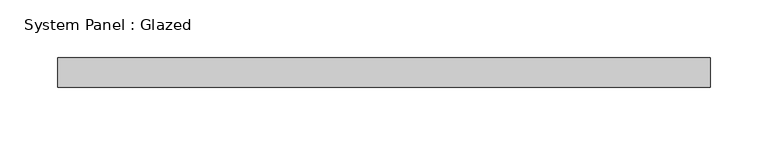
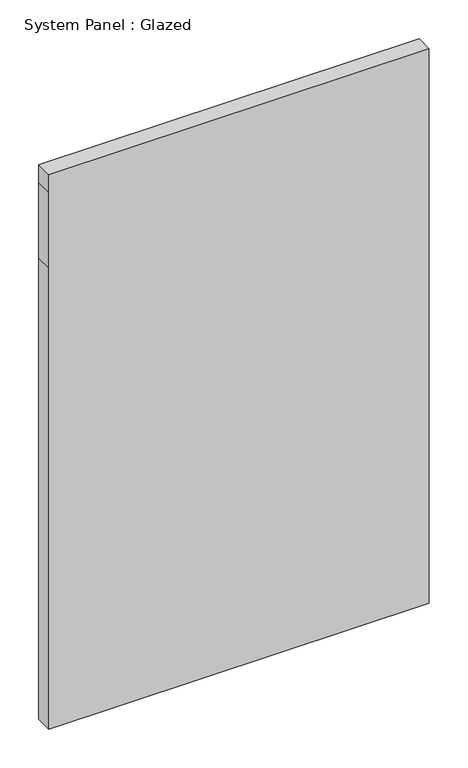
"""IFC4 building model written with IfcOpenShell, lengths in millimetres: plate geometry, System Panel : Glazed."""

from ifc_helpers import new_model, si_unit, frame, origin, place, context, project, spatial, polyline, outline, extrude, source, transform, mapped, element, save


def system_panel_glazed_08392cf6(model_context):
    return source(origin(), model_context, "Body", "SweptSolid", [
        extrude(outline(polyline([(0.0, -282.575), (0.0, 282.575), (723.9, 282.575), (842.4333333, 282.575), (869.95, 282.575), (869.95, -282.575), (842.4333333, -282.575), (723.9, -282.575), (0.0, -282.575)])), frame((0.0, 19.05, 0.0), z_axis=(0.0, 1.0, 0.0), x_axis=(0.0, 0.0, 1.0)), (0.0, 0.0, 1.0), 25.4),
    ])


if __name__ == "__main__":
    model = new_model("IFC4")
    model_context = context("Model", 3, world=origin())
    ifc_project = project(units=[si_unit("LENGTHUNIT", "METRE", prefix="MILLI")], contexts=[model_context])
    site = spatial("IfcSite", under=ifc_project)
    building = spatial("IfcBuilding", under=site)
    placement = place(None, origin())
    system_panel_glazed_shape = system_panel_glazed_08392cf6(model_context)
    element("IfcPlate", 1, ObjectType="System Panel : Glazed", at=placement, inside=building, context=model_context, shape_type="MappedRepresentation", body=[
        mapped(system_panel_glazed_shape, transform((0.0, 0.0, 0.0), x_axis=(1.0, 0.0, 0.0), y_axis=(0.0, 1.0, 0.0), z_axis=(0.0, 0.0, 1.0))),
    ])
    save(model, "model.ifc")

# Revit data of these elements
# Type "System Panel : Glazed"
#   Construction Type Id = "GSP4R"
#   Analytic Construction = "1/8 in Pilkington single glazing"
#   Visual Light Transmittance = 0.9
#   Solar Heat Gain Coefficient = 0.86
#   Heat Transfer Coefficient (U) = 1.18115 BTU/(h·ft²·°F)
#   Define Thermal Properties by = 1
# Element 1 (IfcPlate, "System Panel : Glazed")
#   Materials on its faces: "Glass"
# Materials
#   "Glass": class "Glass", colour RGB 0 128 192, transparency 0.75, Description = "Soda Lime Glass", Cost = 0
